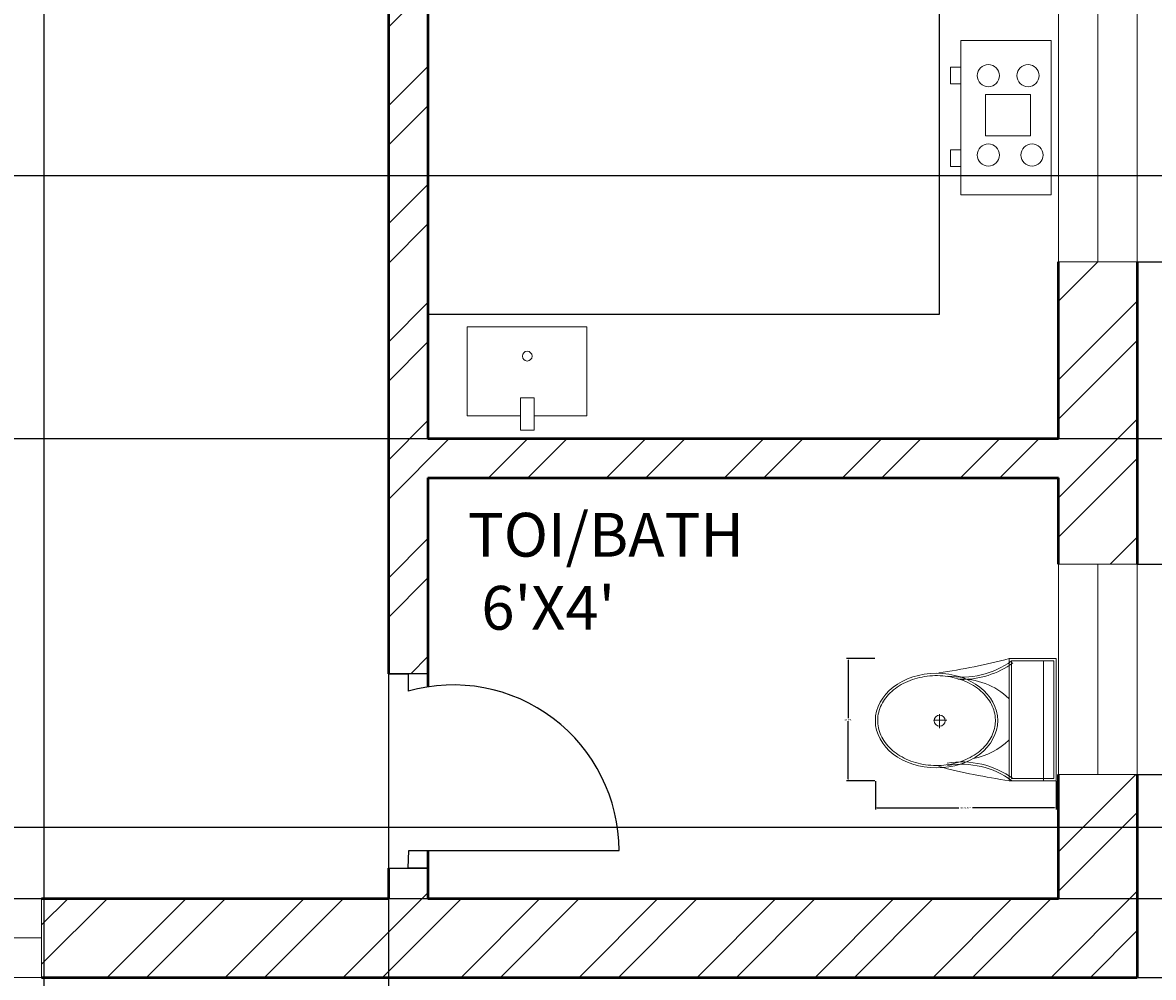
# Model space of a CAD drawing. Units: inches. Extents: x 2310 to 2937, y 1113 to 2410.
# Tile 11 of 23: x 2697 to 2826, y 1737 to 1845. Entities that reach past the tile are written whole.
import ezdxf

# ---------------------------------------------------------------- set-up
doc = ezdxf.new("R2010")
doc.units = ezdxf.units.IN
for name, color, linetype, lineweight in [('A-ANNO-DIMS', 2, 'Continuous', 18), ('A-AREA-IDEN', 7, 'Continuous', 18), ('A-DOOR', 31, 'Continuous', 25), ('A-EQPM', 8, 'Continuous', 18), ('A-FLOR-CASE', 7, 'Continuous', 25), ('A-FLOR-FIXT', 9, 'Continuous', 18), ('A-GLAZ', 191, 'Continuous', 20), ('A-WALL', 7, 'Continuous', 50), ('A-WALL-PATT', 85, 'Continuous', 13)]:
    doc.layers.add(name, color=color, linetype=linetype, lineweight=lineweight)
doc.styles.get("Standard").update_dxf_attribs({"font": 'arial.ttf'})
doc.dimstyles.get("Standard").update_dxf_attribs({"dimtxt": 0.18, "dimasz": 0.18, "dimexe": 0.18, "dimexo": 0.0625, "dimgap": 0.09, "dimtad": 0, "dimtih": 1, "dimtoh": 1, "dimdec": 4, "dimzin": 0, "dimdsep": 46, "dimtxsty": 'Standard', "dimcen": 0.09, "dimadec": 0, "dimazin": 0, "dimtfac": 1, "dimtdec": 4, "dimtofl": 0, "dimtmove": 0, "dimatfit": 3, "dimfxl": 1, "dimtolj": 1, "dimtzin": 0, "dimarcsym": 0})

# ---------------------------------------------------------------- blocks, each defined once
blk = doc.blocks.new('A$C31115884')
for p, q in [((283.1, 497.7), (223.4, 497.7)), ((257.5, 466.4), (257.5, 523.2)), ((0, 200), (0, 0)), ((520, 200), (0, 200)), ((520, 0), (520, 200)), ((10, 190), (10, 10)), ((510, 190), (10, 190)), ((510, 10), (510, 190)), ((510, 54.5), (0, 54.5)), ((10, 10), (510, 10)), ((0, 0), (520, 0))]:
    blk.add_line(p, q)
blk.add_circle((255.6, 496.4), 23.6)
for centre, radius, start, end in [((2777.7, -204.6), 2807, 165.4549, 171.7133), ((3237, 905), 2807, 188.2867, 194.5451), ((-294.5, 403.3), 364.7, 324.2091, 9.3499), ((-294.5, 403.3), 374.7, 324.2091, 9.3499), ((805.8, 403.3), 364.7, 170.6501, 215.7909), ((139.5, 406.2), 293.5, 315.8436, 2.6563), ((805.8, 403.3), 374.7, 179.2036, 215.7909), ((383.6, 406.2), 293.5, 190.2774, 224.1564)]:
    blk.add_arc(centre, radius, start, end)
blk.add_ellipse((256.2, 509.9), major_axis=(0, -260.7), ratio=0.772727)
blk.add_open_spline([(256.2, 259.2), (263.1, 259.2), (270, 259.7), (287.8, 262.3), (298.7, 265.1), (319.9, 273.1), (330.2, 278.4), (350.1, 291.1), (359.7, 298.7), (377.7, 315.9), (386.2, 325.5), (401.7, 346.6), (408.8, 358.1), (421.3, 382.5), (426.8, 395.5), (435.9, 422.4), (439.5, 436.4), (444.8, 465.1), (446.5, 479.7), (447.9, 509.2), (447.6, 524), (445, 553.3), (442.7, 567.8), (436.3, 596), (432.1, 609.7), (421.9, 636), (416, 648.6), (402.5, 672.1), (395, 683), (378.6, 703), (369.8, 712.1), (351.1, 728), (341.3, 734.8), (320.9, 746.2), (310.4, 750.7), (288.9, 757.3), (278, 759.4), (256, 761), (245, 760.6), (223.1, 757.2), (212.3, 754.3), (191.1, 746.1), (180.8, 740.7), (160.9, 727.8), (151.4, 720.1), (133.5, 702.7), (125.1, 693), (109.6, 671.7), (102.6, 660.2), (90.2, 635.7), (84.9, 622.7), (76, 595.6), (72.4, 581.6), (67.2, 552.9), (65.6, 538.2), (64.4, 508.8), (64.8, 494), (67.5, 464.7), (69.9, 450.2), (76.6, 422), (80.8, 408.3), (91.1, 382.2), (97.2, 369.7), (110.8, 346.3), (118.4, 335.4), (134.8, 315.6), (143.7, 306.7), (162.4, 290.9), (172.3, 284.2), (192.8, 273), (203.3, 268.6), (224.8, 262.2), (235.8, 260.2), (249.9, 259.3), (253, 259.2), (256.2, 259.2)], degree=3, knots=[0, 0, 0, 0, 0.110105, 0.110105, 0.285049, 0.285049, 0.459994, 0.459994, 0.634938, 0.634938, 0.809882, 0.809882, 0.984827, 0.984827, 1.159771, 1.159771, 1.334715, 1.334715, 1.50966, 1.50966, 1.684604, 1.684604, 1.859549, 1.859549, 2.034493, 2.034493, 2.209437, 2.209437, 2.384382, 2.384382, 2.559326, 2.559326, 2.73427, 2.73427, 2.909215, 2.909215, 3.084159, 3.084159, 3.259103, 3.259103, 3.434048, 3.434048, 3.608992, 3.608992, 3.783936, 3.783936, 3.958881, 3.958881, 4.133825, 4.133825, 4.30877, 4.30877, 4.483714, 4.483714, 4.658658, 4.658658, 4.833603, 4.833603, 5.008547, 5.008547, 5.183491, 5.183491, 5.358436, 5.358436, 5.53338, 5.53338, 5.708324, 5.708324, 5.883269, 5.883269, 6.058213, 6.058213, 6.233158, 6.233158, 6.283185, 6.283185, 6.283185, 6.283185])
blk = doc.blocks.new('SINK-KITCHEN')
blk.add_lwpolyline([(6.01, 11.79), (7.56, 11.79), (7.56, 8.11), (6.01, 8.11)], close=True)
blk.add_lwpolyline([(7.56, 10.17), (13.64, 10.17), (13.64, 0), (0, 0), (0, 10.17), (6.01, 10.17)])
blk.add_circle((6.79, 3.34), 0.556)
blk = doc.blocks.new('RANGE-4-BURNER')
for points in [[(1.2, 17.61), (1.2, 17.61), (1.2, 17.61), (1.2, 17.61)], [(1.2, 17.61), (11.5, 17.61), (11.5, 0), (1.2, 0)], [(1.2, 14.58), (0, 14.58), (0, 12.67), (1.2, 12.67)], [(4.01, 11.43), (9.13, 11.43), (9.13, 6.73), (4.01, 6.73)], [(1.2, 5.14), (0, 5.14), (0, 3.24), (1.2, 3.24)]]:
    blk.add_lwpolyline(points, close=True)
for centre in [(4.34, 13.6), (8.87, 13.6), (4.34, 4.53), (9.32, 4.53)]:
    blk.add_circle(centre, 1.27)
blk = doc.blocks.new('WIN-24IN')
for p, q in [((0, 24), (9, 24)), ((0, 24), (0, 0)), ((9, 24), (4.5, 24)), ((4.5, 24), (4.5, 0)), ((9, 24), (9, 0)), ((4.5, 0), (0, 0)), ((0, 0), (9, 0))]:
    blk.add_line(p, q)
blk = doc.blocks.new('WIN-36IN')
for p, q in [((4.5, 36), (0, 36)), ((0, 36), (9, 36)), ((0, 36), (0, 0)), ((4.5, 0), (4.5, 36)), ((9, 36), (9, 0)), ((0, 0), (9, 0)), ((9, 0), (4.5, 0))]:
    blk.add_line(p, q)
blk = doc.blocks.new('WIN-60IN')
for p, q in [((4.5, 60), (0, 60)), ((0, 60), (9, 60)), ((0, 60), (0, 0)), ((4.5, 0), (4.5, 60)), ((9, 60), (9, 0)), ((0, 0), (9, 0)), ((9, 0), (4.5, 0))]:
    blk.add_line(p, q)
blk = doc.blocks.new('*D21')
at = {"layer": 'A-ANNO-DIMS', "color": 0, "lineweight": -2, "transparency": 16777216}
for p, q in [((2794.08, 1758.89), (2794.08, 1755.68)), ((2814.73, 1758.89), (2814.73, 1755.68)), ((2794.26, 1755.86), (2803.63, 1755.86)), ((2814.55, 1755.86), (2805.18, 1755.86))]:
    blk.add_line(p, q, dxfattribs=at)
at = {"layer": 'A-ANNO-DIMS', "color": 0, "transparency": 16777216}
for points in [[(2794.26, 1755.89), (2794.26, 1755.83), (2794.08, 1755.86)], [(2814.55, 1755.89), (2814.55, 1755.83), (2814.73, 1755.86)]]:
    blk.add_solid(points, dxfattribs=at)
at = {"layer": 'Defpoints', "color": 0, "transparency": 16777216}
for p in [(2794.08, 1758.96), (2814.73, 1758.96), (2794.08, 1755.86)]:
    blk.add_point(p, dxfattribs=at)
at = {"layer": 'A-ANNO-DIMS', "color": 0, "transparency": 16777216, "insert": (2804.41, 1755.86), "char_height": 0.18, "attachment_point": 5}
blk.add_mtext('\\A1;WC 21 TYP.', dxfattribs=at)
blk = doc.blocks.new('*D22')
at = {"layer": 'A-ANNO-DIMS', "color": 0, "lineweight": -2, "transparency": 16777216}
for p, q in [((2794.02, 1772.89), (2790.8, 1772.89)), ((2790.98, 1772.71), (2790.98, 1766.1)), ((2790.98, 1759.14), (2790.98, 1765.74)), ((2794.02, 1758.96), (2790.8, 1758.96))]:
    blk.add_line(p, q, dxfattribs=at)
at = {"layer": 'A-ANNO-DIMS', "color": 0, "transparency": 16777216}
for points in [[(2790.95, 1772.71), (2791.01, 1772.71), (2790.98, 1772.89)], [(2790.95, 1759.14), (2791.01, 1759.14), (2790.98, 1758.96)]]:
    blk.add_solid(points, dxfattribs=at)
at = {"layer": 'Defpoints', "color": 0, "transparency": 16777216}
for p in [(2790.98, 1772.89), (2794.08, 1772.89), (2794.08, 1758.96)]:
    blk.add_point(p, dxfattribs=at)
at = {"layer": 'A-ANNO-DIMS', "color": 0, "transparency": 16777216, "insert": (2790.98, 1765.92), "char_height": 0.18, "attachment_point": 5}
blk.add_mtext('\\A1;14 TYP.', dxfattribs=at)
blk = doc.blocks.new('*D42')
at = {"layer": 'A-ANNO-DIMS', "color": 0, "lineweight": -2, "transparency": 16777216}
for p, q in [((2699.14, 2347.45), (2699.14, 1649.5)), ((2738.49, 2347.45), (2738.49, 1649.5)), ((2699.32, 1649.68), (2718.42, 1649.68)), ((2738.31, 1649.68), (2719.21, 1649.68))]:
    blk.add_line(p, q, dxfattribs=at)
at = {"layer": 'A-ANNO-DIMS', "color": 0, "transparency": 16777216}
for points in [[(2699.32, 1649.71), (2699.32, 1649.65), (2699.14, 1649.68)], [(2738.31, 1649.71), (2738.31, 1649.65), (2738.49, 1649.68)]]:
    blk.add_solid(points, dxfattribs=at)
at = {"layer": 'Defpoints', "color": 0, "transparency": 16777216}
for p in [(2699.14, 2347.51), (2738.49, 2347.51), (2738.49, 1649.68)]:
    blk.add_point(p, dxfattribs=at)
at = {"layer": 'A-ANNO-DIMS', "color": 0, "transparency": 16777216, "insert": (2718.81, 1649.68), "char_height": 0.18, "attachment_point": 5}
blk.add_mtext('\\A1;39.35', dxfattribs=at)
blk = doc.blocks.new('*D45')
at = {"layer": 'A-ANNO-DIMS', "color": 0, "lineweight": -2, "transparency": 16777216}
for p, q in [((2824.05, 1759.67), (2858.02, 1759.67)), ((2857.84, 1759.49), (2857.84, 1748.27)), ((2857.84, 1736.69), (2857.84, 1747.91)), ((2824.05, 1736.51), (2858.02, 1736.51))]:
    blk.add_line(p, q, dxfattribs=at)
at = {"layer": 'A-ANNO-DIMS', "color": 0, "transparency": 16777216}
for points in [[(2857.81, 1759.49), (2857.87, 1759.49), (2857.84, 1759.67)], [(2857.81, 1736.69), (2857.87, 1736.69), (2857.84, 1736.51)]]:
    blk.add_solid(points, dxfattribs=at)
at = {"layer": 'Defpoints', "color": 0, "transparency": 16777216}
for p in [(2823.99, 1759.67), (2857.84, 1759.67), (2823.99, 1736.51)]:
    blk.add_point(p, dxfattribs=at)
at = {"layer": 'A-ANNO-DIMS', "color": 0, "transparency": 16777216, "insert": (2857.84, 1748.09), "char_height": 0.18, "attachment_point": 5}
blk.add_mtext('\\A1;23.154', dxfattribs=at)
blk = doc.blocks.new('*D46')
at = {"layer": 'A-ANNO-DIMS', "color": 0, "lineweight": -2, "transparency": 16777216}
for p, q in [((2824.05, 1818.17), (2858.02, 1818.17)), ((2857.84, 1817.99), (2857.84, 1801.1)), ((2857.84, 1783.85), (2857.84, 1800.74)), ((2824.05, 1783.67), (2858.02, 1783.67))]:
    blk.add_line(p, q, dxfattribs=at)
at = {"layer": 'A-ANNO-DIMS', "color": 0, "transparency": 16777216}
for points in [[(2857.81, 1817.99), (2857.87, 1817.99), (2857.84, 1818.17)], [(2857.81, 1783.85), (2857.87, 1783.85), (2857.84, 1783.67)]]:
    blk.add_solid(points, dxfattribs=at)
at = {"layer": 'Defpoints', "color": 0, "transparency": 16777216}
for p in [(2823.99, 1818.17), (2857.84, 1818.17), (2823.99, 1783.67)]:
    blk.add_point(p, dxfattribs=at)
at = {"layer": 'A-ANNO-DIMS', "color": 0, "transparency": 16777216, "insert": (2857.84, 1800.92), "char_height": 0.18, "attachment_point": 5}
blk.add_mtext('\\A1;34.5', dxfattribs=at)
blk = doc.blocks.new('*D55')
at = {"layer": 'A-ANNO-DIMS', "color": 0, "lineweight": -2, "transparency": 16777216}
for p, q in [((2403.55, 1753.64), (2858.02, 1753.64)), ((2857.84, 1753.46), (2857.84, 1749.76)), ((2857.84, 1745.69), (2857.84, 1749.4)), ((2403.55, 1745.51), (2858.02, 1745.51))]:
    blk.add_line(p, q, dxfattribs=at)
at = {"layer": 'A-ANNO-DIMS', "color": 0, "transparency": 16777216}
for points in [[(2857.81, 1753.46), (2857.87, 1753.46), (2857.84, 1753.64)], [(2857.81, 1745.69), (2857.87, 1745.69), (2857.84, 1745.51)]]:
    blk.add_solid(points, dxfattribs=at)
at = {"layer": 'Defpoints', "color": 0, "transparency": 16777216}
for p in [(2403.49, 1753.64), (2857.84, 1753.64), (2403.49, 1745.51)]:
    blk.add_point(p, dxfattribs=at)
at = {"layer": 'A-ANNO-DIMS', "color": 0, "transparency": 16777216, "insert": (2857.84, 1749.58), "char_height": 0.18, "attachment_point": 5}
blk.add_mtext('\\A1;8.127', dxfattribs=at)
blk = doc.blocks.new('*D56')
at = {"layer": 'A-ANNO-DIMS', "color": 0, "lineweight": -2, "transparency": 16777216}
for p, q in [((2403.55, 1828.04), (2858.02, 1828.04)), ((2857.84, 1827.86), (2857.84, 1813.21)), ((2857.84, 1798.19), (2857.84, 1812.85)), ((2403.55, 1798.01), (2858.02, 1798.01))]:
    blk.add_line(p, q, dxfattribs=at)
at = {"layer": 'A-ANNO-DIMS', "color": 0, "transparency": 16777216}
for points in [[(2857.81, 1827.86), (2857.87, 1827.86), (2857.84, 1828.04)], [(2857.81, 1798.19), (2857.87, 1798.19), (2857.84, 1798.01)]]:
    blk.add_solid(points, dxfattribs=at)
at = {"layer": 'Defpoints', "color": 0, "transparency": 16777216}
for p in [(2403.49, 1828.04), (2857.84, 1828.04), (2403.49, 1798.01)]:
    blk.add_point(p, dxfattribs=at)
at = {"layer": 'A-ANNO-DIMS', "color": 0, "transparency": 16777216, "insert": (2857.84, 1813.03), "char_height": 0.18, "attachment_point": 5}
blk.add_mtext('\\A1;30.03', dxfattribs=at)
blk = doc.blocks.new('*D58')
at = {"layer": 'A-ANNO-DIMS', "color": 0, "lineweight": -2, "transparency": 16777216}
for p, q in [((2475.55, 1882.51), (2858.02, 1882.51)), ((2857.84, 1882.33), (2857.84, 1840.45)), ((2857.84, 1798.19), (2857.84, 1840.08)), ((2475.55, 1798.01), (2858.02, 1798.01))]:
    blk.add_line(p, q, dxfattribs=at)
at = {"layer": 'A-ANNO-DIMS', "color": 0, "transparency": 16777216}
for points in [[(2857.81, 1882.33), (2857.87, 1882.33), (2857.84, 1882.51)], [(2857.81, 1798.19), (2857.87, 1798.19), (2857.84, 1798.01)]]:
    blk.add_solid(points, dxfattribs=at)
at = {"layer": 'Defpoints', "color": 0, "transparency": 16777216}
for p in [(2475.49, 1882.51), (2857.84, 1882.51), (2475.49, 1798.01)]:
    blk.add_point(p, dxfattribs=at)
at = {"layer": 'A-ANNO-DIMS', "color": 0, "transparency": 16777216, "insert": (2857.84, 1840.26), "char_height": 0.18, "attachment_point": 5}
blk.add_mtext('\\A1;84.5', dxfattribs=at)

msp = doc.modelspace()

# ---------------------------------------------------------------- hatches: boundary and pattern name
at = {"layer": 'A-WALL-PATT'}
h = msp.add_hatch(dxfattribs=at)
h.set_pattern_fill('ANSI32', color=256)
h.paths.add_polyline_path([(2639.1394, 2356.5139), (2563.662, 2356.5139), (2563.662, 2347.5139), (2606.9859, 2347.5139), (2606.9859, 2210.5139), (2514.2692, 2210.5139), (2514.2692, 2206.0139), (2606.9859, 2206.0139), (2606.9859, 2098.0139), (2602.689, 2098.0139), (2602.689, 2093.5139), (2615.5262, 2093.5139), (2615.5262, 2095.7639), (2615.5262, 2098.0139), (2611.4859, 2098.0139), (2611.4859, 2206.0139), (2703.9391, 2206.0139), (2703.9391, 2208.2639), (2703.9391, 2210.5139), (2611.4859, 2210.5139), (2611.4859, 2347.5139), (2639.1394, 2347.5139)])
h.paths.add_polyline_path([(2823.9859, 2356.5139), (2699.1394, 2356.5139), (2699.1394, 2347.5139), (2738.4859, 2347.5139), (2738.4859, 2343.9266), (2742.9859, 2343.9266), (2742.9859, 2347.5139), (2814.9859, 2347.5139), (2814.9859, 2336.76), (2823.9859, 2336.76)])
h.paths.add_polyline_path([(2823.9859, 2312.76), (2814.9859, 2312.76), (2814.9859, 2299.5139), (2742.9859, 2299.5139), (2742.9859, 2323.0159), (2740.7359, 2323.0159), (2738.4859, 2323.0159), (2738.4859, 2210.5139), (2734.5483, 2210.5139), (2734.5483, 2206.0139), (2746.8769, 2206.0139), (2746.8769, 2208.2639), (2746.8769, 2210.5139), (2742.9859, 2210.5139), (2742.9859, 2295.0139), (2814.9859, 2295.0139), (2814.9859, 2269.8977), (2823.9859, 2269.8977)])
h.paths.add_polyline_path([(2823.9859, 2210.5139), (2823.9859, 2233.8977), (2819.4859, 2233.8977), (2814.9859, 2233.8977), (2814.9859, 2210.5139), (2769.9745, 2210.5139), (2769.9745, 2206.0139), (2814.9859, 2206.0139), (2814.9859, 2178.3027), (2823.9859, 2178.3027)])
h.paths.add_polyline_path([(2823.9859, 2118.3027), (2819.4859, 2118.3027), (2814.9859, 2118.3027), (2814.9859, 2098.0139), (2647.0333, 2098.0139), (2647.0333, 2093.5139), (2814.9859, 2093.5139), (2814.9859, 1999.5139), (2650.6052, 1999.5139), (2650.6052, 1995.0139), (2814.9859, 1995.0139), (2814.9859, 1969.9784), (2823.9859, 1969.9784)])
h.paths.add_polyline_path([(2403.4859, 2093.5139), (2569.9888, 2093.5139), (2569.9888, 2095.7639), (2569.9888, 2098.0139), (2403.4859, 2098.0139), (2403.4859, 2131.7587), (2394.4859, 2131.7587), (2394.4859, 1967.522), (2403.4859, 1967.522), (2403.4859, 1995.0139), (2569.8903, 1995.0139), (2569.8903, 1997.2639), (2569.8903, 1999.5139), (2403.4859, 1999.5139)])
h.paths.add_polyline_path([(2503.662, 2356.5139), (2394.4859, 2356.5139), (2394.4859, 2337.9231), (2398.9859, 2337.9231), (2403.4859, 2337.9231), (2403.4859, 2347.5139), (2475.4859, 2347.5139), (2475.4859, 2343.0384), (2479.9859, 2343.0384), (2479.9859, 2347.5139), (2503.662, 2347.5139)])
h.paths.add_polyline_path([(2498.3065, 1745.5139), (2479.9859, 1745.5139), (2479.9859, 1749.1663), (2477.7359, 1749.1663), (2475.4859, 1749.1663), (2475.4859, 1745.5139), (2403.4859, 1745.5139), (2403.4859, 1753.6409), (2398.9859, 1753.6409), (2394.4859, 1753.6409), (2394.4859, 1736.5139), (2498.3065, 1736.5139), (2498.3065, 1741.0139)])
h.paths.add_polyline_path([(2479.9859, 1882.5139), (2483.9367, 1882.5139), (2483.9367, 1887.0139), (2471.5501, 1887.0139), (2471.5501, 1885.1969), (2471.5501, 1882.5139), (2475.4859, 1882.5139), (2475.4859, 1798.0139), (2403.4859, 1798.0139), (2403.4859, 1828.0433), (2402.2852, 1828.0433), (2394.4859, 1828.0433), (2394.4859, 1777.6409), (2403.4859, 1777.6409), (2403.4859, 1793.5139), (2475.4859, 1793.5139), (2475.4859, 1769.1696), (2479.9859, 1769.1696)])
h.paths.add_polyline_path([(2403.4859, 1907.522), (2398.9859, 1907.522), (2394.4859, 1907.522), (2394.4859, 1864.0433), (2403.4859, 1864.0433), (2403.4859, 1882.5139), (2448.9325, 1882.5139), (2448.9325, 1884.7639), (2448.9325, 1887.0139), (2403.4859, 1887.0139)])
h.paths.add_polyline_path([(2702.2061, 1887.0139), (2611.4859, 1887.0139), (2611.4859, 1995.0139), (2615.6132, 1995.0139), (2615.6132, 1999.5139), (2602.4798, 1999.5139), (2602.4798, 1997.2639), (2602.4798, 1995.0139), (2606.9859, 1995.0139), (2606.9859, 1887.0139), (2516.2443, 1887.0139), (2516.2443, 1884.7639), (2516.2443, 1882.5139), (2606.9859, 1882.5139), (2606.9859, 1745.5139), (2558.3065, 1745.5139), (2558.3065, 1736.5139), (2638.8921, 1736.5139), (2638.8921, 1741.0139), (2638.8921, 1745.5139), (2611.4859, 1745.5139), (2611.4859, 1882.5139), (2702.2061, 1882.5139)])
h.paths.add_polyline_path([(2823.9859, 1909.9784), (2819.4859, 1909.9784), (2814.9859, 1909.9784), (2814.9859, 1887.0139), (2769.144, 1887.0139), (2769.144, 1884.7639), (2769.144, 1882.5139), (2814.9859, 1882.5139), (2814.9859, 1854.1704), (2823.9859, 1854.1704)])
h.paths.add_polyline_path([(2823.9859, 1818.1704), (2819.4859, 1818.1704), (2814.9859, 1818.1704), (2814.9859, 1798.0139), (2742.9859, 1798.0139), (2742.9859, 1882.5139), (2746.805, 1882.5139), (2746.805, 1887.0139), (2733.7334, 1887.0139), (2733.7334, 1884.7639), (2733.7334, 1882.5139), (2738.4859, 1882.5139), (2738.4859, 1771.1728), (2740.7359, 1771.1728), (2742.9859, 1771.1728), (2742.9859, 1793.5139), (2814.9859, 1793.5139), (2814.9859, 1783.6684), (2823.9859, 1783.6684)])
h.paths.add_polyline_path([(2823.9859, 1759.6684), (2814.9859, 1759.6684), (2814.9859, 1745.5139), (2742.9859, 1745.5139), (2742.9859, 1748.9831), (2740.7359, 1748.9831), (2738.4859, 1748.9831), (2738.4859, 1745.5139), (2698.8921, 1745.5139), (2698.8921, 1736.5139), (2823.9859, 1736.5139)])

# ---------------------------------------------------------------- linework, layer by layer
at = {"layer": 'A-DOOR'}
for p, q in [((2742.9859, 1771.1728), (2738.4859, 1771.1728)), ((2738.4859, 1771.1728), (2740.7359, 1771.1728)), ((2740.7359, 1771.1728), (2740.7359, 1769.1728)), ((2738.4859, 1768.8626), (2738.4859, 1768.8626)), ((2740.7359, 1748.9831), (2740.8143, 1750.9816)), ((2740.8143, 1750.9816), (2764.8143, 1750.9816)), ((2738.4859, 1748.9831), (2742.9859, 1748.9831)), ((2742.9859, 1748.9831), (2740.7359, 1748.9831))]:
    msp.add_line(p, q, dxfattribs=at)
msp.add_arc((2745.9034, 1750.9816), 18.9109, 360, 105.857766, dxfattribs=at)
at = {"layer": 'A-FLOR-CASE'}
for p, q in [((2801.3852, 1882.5139), (2801.3852, 1812.1659)), ((2801.3852, 1812.1659), (2742.9859, 1812.1659))]:
    msp.add_line(p, q, dxfattribs=at)
at = {"layer": 'A-GLAZ'}
msp.add_line((2823.9859, 1759.6684), (2823.9859, 1759.6684), dxfattribs=at)
at = {"layer": 'A-WALL'}
for p, q in [((2738.4859, 1882.5139), (2738.4859, 1771.1728)), ((2742.9859, 1882.5139), (2742.9859, 1798.0139)), ((2814.9859, 1798.0139), (2814.9859, 1818.1704)), ((2823.9859, 1818.1704), (2823.9859, 1783.6684)), ((2742.9859, 1798.0139), (2814.9859, 1798.0139)), ((2742.9859, 1793.5139), (2814.9859, 1793.5139)), ((2742.9859, 1793.5139), (2742.9859, 1769.6661)), ((2814.9859, 1783.6684), (2814.9859, 1793.5139)), ((2814.9859, 1745.5139), (2814.9859, 1759.6684)), ((2823.9859, 1759.6684), (2823.9859, 1736.5139)), ((2742.9859, 1750.9816), (2742.9859, 1745.5139)), ((2738.4859, 1748.9831), (2738.4859, 1745.5139)), ((2698.8921, 1745.5139), (2738.4859, 1745.5139)), ((2742.9859, 1745.5139), (2814.9859, 1745.5139)), ((2698.8921, 1736.5139), (2823.9859, 1736.5139))]:
    msp.add_line(p, q, dxfattribs=at)

# ---------------------------------------------------------------- block references
at = {"layer": 'A-EQPM'}
msp.add_blockref('RANGE-4-BURNER', (2802.647, 1825.8353), dxfattribs=at)
msp.add_blockref('RANGE-4-BURNER', (2802.647, 1825.8353), dxfattribs=at)
at = {"layer": 'A-FLOR-FIXT', "rotation": 180}
msp.add_blockref('SINK-KITCHEN', (2761.1247, 1810.7577), dxfattribs=at)
msp.add_blockref('SINK-KITCHEN', (2761.1247, 1810.7577), dxfattribs=at)
at = {"layer": 'A-FLOR-FIXT', "xscale": 0.0268011493576733, "yscale": 0.0268011493576733, "zscale": 0.0268011493576733, "rotation": 89.99999999999999}
msp.add_blockref('A$C31115884', (2814.733, 1758.9563), dxfattribs=at)
msp.add_blockref('A$C31115884', (2814.733, 1758.9563), dxfattribs=at)
at = {"layer": 'A-GLAZ'}
for name, p in [('WIN-36IN', (2814.9859, 1818.1704)), ('WIN-24IN', (2814.9859, 1759.6684))]:
    msp.add_blockref(name, p, dxfattribs=at)
at = {"layer": 'A-GLAZ', "rotation": 270}
msp.add_blockref('WIN-60IN', (2638.8921, 1745.5139), dxfattribs=at)

# ---------------------------------------------------------------- texts
at = {"layer": 'A-AREA-IDEN', "insert": (2742.9859, 1789.5308), "char_height": 5, "attachment_point": 1}
msp.add_mtext_dynamic_manual_height_columns("   TOI/BATH\\P    6'X4'", width=161.794338, gutter_width=12.5, heights=[0], dxfattribs=at)

# ---------------------------------------------------------------- dimensions: what is measured, and where the dimension line sits
at = {"layer": 'A-ANNO-DIMS'}
dim = msp.add_linear_dim(base=(2738.4859, 1649.6807), p1=(2699.1394, 2347.5139), p2=(2738.4859, 2347.5139), dimstyle='Standard', override={"dimdec": 2, "dimlfac": 1, "dimrnd": 0, "dimzin": 0, "dimdsep": 46, "dimlunit": 2}, dxfattribs=at)
dim.commit()
dim.dimension.update_dxf_attribs({"geometry": '*D42', "text_midpoint": (2718.8127, 1649.6807)})
for base, p1, p2, override, picture, middle in [((2857.8359, 1882.5139), (2475.4859, 1798.0139), (2475.4859, 1882.5139), {"dimdec": 1, "dimlfac": 1, "dimrnd": 0, "dimzin": 0, "dimdsep": 46, "dimlunit": 2}, '*D58', (2857.8359, 1840.2639)), ((2857.8359, 1828.0433), (2403.4859, 1798.0139), (2403.4859, 1828.0433), {"dimdec": 2, "dimlfac": 1, "dimrnd": 0, "dimzin": 0, "dimdsep": 46, "dimlunit": 2}, '*D56', (2857.8359, 1813.0286)), ((2857.8359, 1818.1704), (2823.9859, 1783.6684), (2823.9859, 1818.1704), {"dimdec": 1, "dimlfac": 1, "dimrnd": 0, "dimzin": 0, "dimdsep": 46, "dimlunit": 2}, '*D46', (2857.8359, 1800.9194)), ((2857.83594, 1759.66842), (2823.98594, 1736.51394), (2823.98594, 1759.66842), {"dimdec": 3, "dimlfac": 1, "dimrnd": 0, "dimzin": 0, "dimdsep": 46, "dimlunit": 2}, '*D45', (2857.83594, 1748.09118)), ((2857.8359, 1753.6409), (2403.4859, 1745.5139), (2403.4859, 1753.6409), {"dimdec": 3, "dimlfac": 1, "dimrnd": 0, "dimzin": 0, "dimdsep": 46, "dimlunit": 2}, '*D55', (2857.8359, 1749.5774))]:
    dim = msp.add_linear_dim(base=base, p1=p1, p2=p2, angle=90, dimstyle='Standard', override=override, dxfattribs=at)
    dim.commit()
    dim.dimension.update_dxf_attribs({"geometry": picture, "text_midpoint": middle})
for base, p1, p2, angle, text, picture, middle in [((2790.983, 1772.8929), (2794.0809, 1758.9563), (2794.0809, 1772.8929), 90, '<> TYP.', '*D22', (2790.983, 1765.9246)), ((2794.0809, 1755.8584), (2814.733, 1758.9563), (2794.0809, 1758.9563), 180, 'WC <> TYP.', '*D21', (2804.4069, 1755.8584))]:
    dim = msp.add_linear_dim(base=base, p1=p1, p2=p2, angle=angle, text=text, dimstyle='Standard', override={"dimdec": 0, "dimlfac": 1, "dimrnd": 0, "dimzin": 0, "dimdsep": 46, "dimlunit": 2}, dxfattribs=at)
    dim.commit()
    dim.dimension.update_dxf_attribs({"geometry": picture, "text_midpoint": middle})

doc.saveas('drawing.dxf')
